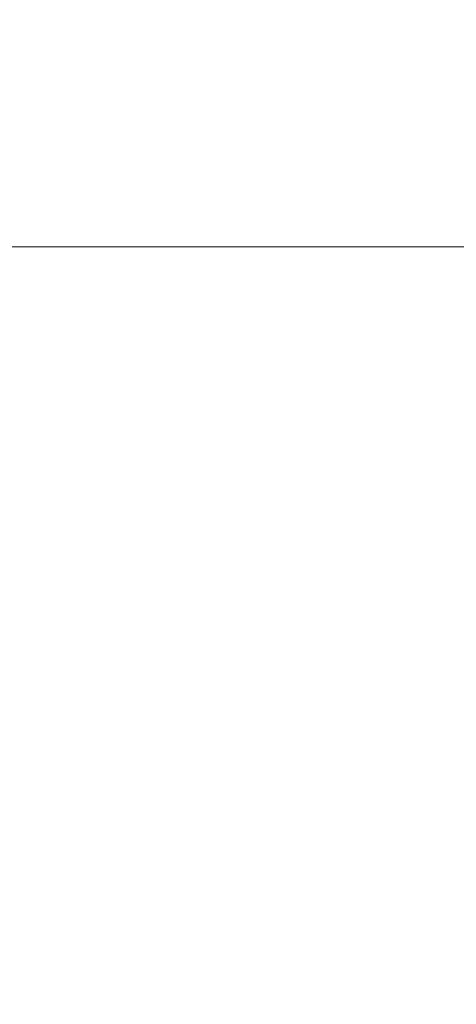
# Model space of a CAD drawing. Units: millimetres. Extents: x 595116 to 630915, y 909473 to 920225.
# Tile 76 of 134: x 629619 to 629628, y 919286 to 919307. Entities that reach past the tile are written whole.
import ezdxf

# ---------------------------------------------------------------- set-up
doc = ezdxf.new("R2010")
doc.units = ezdxf.units.MM
doc.layers.add('Dimension', color=3, linetype='Continuous', lineweight=18)
doc.layers.add('L-PLNT', color=85, linetype='Continuous', lineweight=13)
doc.styles.get("Standard").update_dxf_attribs({"font": 'arial.ttf'})
doc.dimstyles.new('ISO-25', dxfattribs={"dimtxt": 9, "dimasz": 6, "dimexe": 1.25, "dimexo": 0.625, "dimtad": 1, "dimlunit": 4, "dimtxsty": 'Standard', "dimcen": 2.5, "dimadec": 0, "dimazin": 0, "dimtfac": 1, "dimtmove": 0, "dimatfit": 3, "dimfxl": 1, "dimarcsym": 0})

# ---------------------------------------------------------------- blocks, each defined once
blk = doc.blocks.new('*D216')
at = {"layer": 'Defpoints', "color": 0, "transparency": 16777216}
for p in [(629743.541, 919411.928), (629505.041, 919411.828), (629743.541, 918832.378)]:
    blk.add_point(p, dxfattribs=at)
at = {"layer": 'Dimension', "color": 0, "lineweight": -2, "transparency": 16777216}
for p, q in [((629743.541, 919411.303), (629743.541, 918831.128)), ((629505.041, 919411.203), (629505.041, 918831.128)), ((629511.041, 918832.378), (629737.541, 918832.378))]:
    blk.add_line(p, q, dxfattribs=at)
at = {"layer": 'Dimension', "color": 0, "transparency": 16777216}
for points in [[(629511.041, 918833.378), (629511.041, 918831.378), (629505.041, 918832.378)], [(629737.541, 918833.378), (629737.541, 918831.378), (629743.541, 918832.378)]]:
    blk.add_solid(points, dxfattribs=at)
at = {"layer": 'Dimension', "color": 0, "transparency": 16777216, "insert": (629624.291, 918837.656), "char_height": 9, "attachment_point": 5}
blk.add_mtext('19\'-10 1/2"', dxfattribs=at)
blk = doc.blocks.new('*D220')
at = {"layer": 'Defpoints', "color": 0, "transparency": 16777216}
for p in [(629824.951, 920160.756), (629511.274, 919302.009), (629824.951, 919302.009)]:
    blk.add_point(p, dxfattribs=at)
at = {"layer": 'Dimension', "color": 0, "lineweight": -2, "transparency": 16777216}
for p, q in [((629511.274, 919302.634), (629511.274, 920162.006)), ((629824.951, 919302.634), (629824.951, 920162.006)), ((629517.274, 920160.756), (629818.951, 920160.756))]:
    blk.add_line(p, q, dxfattribs=at)
at = {"layer": 'Dimension', "color": 0, "transparency": 16777216}
for points in [[(629517.274, 920161.756), (629517.274, 920159.756), (629511.274, 920160.756)], [(629818.951, 920161.756), (629818.951, 920159.756), (629824.951, 920160.756)]]:
    blk.add_solid(points, dxfattribs=at)
at = {"layer": 'Dimension', "color": 0, "transparency": 16777216, "insert": (629668.113, 920166.035), "char_height": 9, "attachment_point": 5}
blk.add_mtext('26\'-1 1/2"', dxfattribs=at)

msp = doc.modelspace()

# ---------------------------------------------------------------- linework, layer by layer
at = {"layer": 'L-PLNT'}
msp.add_line((629824.951, 919302.009), (629511.274, 919302.009), dxfattribs=at)

# ---------------------------------------------------------------- dimensions: what is measured, and where the dimension line sits
at = {"layer": 'Dimension'}
for base, p1, p2, picture, middle in [((629824.951, 920160.756), (629511.274, 919302.009), (629824.951, 919302.009), '*D220', (629668.113, 920166.035)), ((629743.541, 918832.378), (629505.041, 919411.828), (629743.541, 919411.928), '*D216', (629624.291, 918837.656))]:
    dim = msp.add_linear_dim(base=base, p1=p1, p2=p2, dimstyle='ISO-25', override={"dimdec": 1, "dimlfac": 1, "dimrnd": 0, "dimzin": 1, "dimdsep": 46, "dimlunit": 4, "dimfrac": 2}, dxfattribs=at)
    dim.commit()
    dim.dimension.update_dxf_attribs({"geometry": picture, "text_midpoint": middle})

doc.saveas('drawing.dxf')
